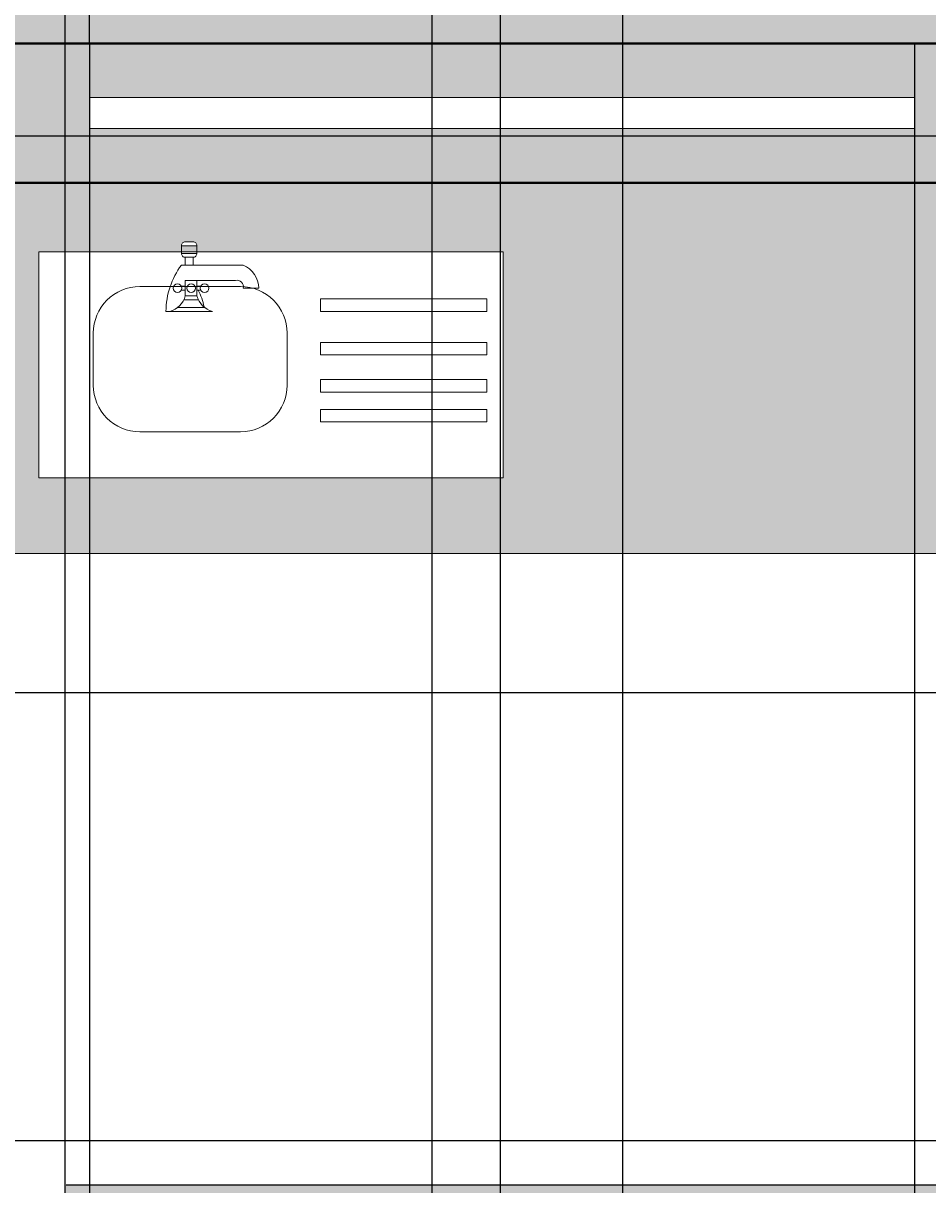
# Model space of a CAD drawing. Units: inches. Extents: x 818 to 1898, y 976 to 2364.
# Tile 85 of 96: x 1481 to 1539, y 1979 to 2054. Entities that reach past the tile are written whole.
import ezdxf

# ---------------------------------------------------------------- set-up
doc = ezdxf.new("R2010")
doc.units = ezdxf.units.IN
doc.header["$LTSCALE"] = 5
doc.header["$MEASUREMENT"] = 0
for name, color, linetype, lineweight in [('A-ANNO-DIMS', 2, 'Continuous', 18), ('A-FLOR-CASE', 8, 'Continuous', 18), ('A-FLOR-FIXT', 9, 'Continuous', 18), ('A-FURN-PATT', 8, 'Continuous', 9), ('A-GLAZ', 4, 'Continuous', 18), ('A-WALL', 7, 'Continuous', 40)]:
    doc.layers.add(name, color=color, linetype=linetype, lineweight=lineweight)
for name, color, linetype, lineweight, true_color in [('A-GLAZ-PATT', 141, 'Continuous', 9, 0xadddf7), ('A-WALL-PATT', 251, 'Continuous', 13, 0x636466), ('L-PLNT-PATT', 114, 'Continuous', 9, 0x139b48)]:
    doc.layers.add(name, color=color, linetype=linetype, lineweight=lineweight, true_color=true_color)
doc.styles.get("Standard").update_dxf_attribs({"font": 'arial.ttf'})
doc.dimstyles.get("Standard").update_dxf_attribs({"dimtxt": 0.18, "dimasz": 0.18, "dimexe": 0.18, "dimexo": 0.0625, "dimgap": 0.09, "dimtad": 0, "dimtih": 1, "dimtoh": 1, "dimdec": 4, "dimzin": 0, "dimdsep": 46, "dimtxsty": 'Standard', "dimcen": 0.09, "dimadec": 0, "dimazin": 0, "dimtfac": 1, "dimtdec": 4, "dimtofl": 0, "dimtmove": 0, "dimatfit": 3, "dimfxl": 1, "dimtolj": 1, "dimtzin": 0, "dimarcsym": 0})

# ---------------------------------------------------------------- blocks, each defined once
blk = doc.blocks.new('Faucet - Bathroom side')
for p, q in [((-0.625, 4.25), (0.375, 4.25)), ((0.375, 3.75), (-0.625, 3.75)), ((-0.375, 3), (-0.375, 3.5)), ((0.125, 3.5), (0.125, 3)), ((-0.625, 3), (3.375, 3)), ((-0.375, 1.625), (-0.625, 1.625)), ((2.875, 2), (0.375, 2)), ((0.375, 1.625), (0.625, 1.625)), ((-0.375, 1.375), (-0.625, 1.375)), ((0.375, 1.375), (0.625, 1.375)), ((4.375, 1.5), (3.375, 1.5)), ((-1.625, 0), (-1.375, 0)), ((-1.375, 0), (1.375, 0)), ((-0.88366, 0.25), (0.88424, 0.25)), ((0.48078, 0.75), (-0.47286, 0.75))]:
    blk.add_line(p, q)
for points in [[(-0.625, 3.75), (-0.625, 4.25)], [(-0.375, 4.5), (0.125, 4.5)], [(0.375, 4.25), (0.375, 3.75)], [(0.125, 3.5), (-0.375, 3.5)]]:
    blk.add_lwpolyline(points)
blk.add_lwpolyline([(-0.375, 1), (-0.375, 2), (0.375, 2), (0.375, 1)], close=True)
for centre in [(-0.875, 1.5), (0, 1.5), (0.875, 1.5)]:
    blk.add_circle(centre, 0.27951)
for centre, radius, start, end in [((-0.38253, 4.2575), 0.24259, 88.22243, 181.7776), ((0.13252, 4.2575), 0.24259, 358.2224, 91.77757), ((-0.38253, 3.7424), 0.24259, 178.2224, 271.7776), ((0.13252, 3.7424), 0.24259, 268.2224, 1.777565), ((3.45929, -0.0281), 5.08436, 143.4467, 179.6834), ((2.70708, 1.4714), 1.66816, 0.9827695, 66.39737), ((2.96867, 1.5936), 0.41699, 347.0192, 102.9808), ((-1.75, 1.375), 1.42522, 285.2551, 344.7449), ((1.75, 1.375), 1.42522, 195.2551, 254.7449), ((-2.49562, -0.286), 3.38273, 9.709485, 29.48735)]:
    blk.add_arc(centre, radius, start, end)
blk = doc.blocks.new('*D73')
at = {"layer": 'A-ANNO-DIMS', "color": 0, "lineweight": -2, "ltscale": 5, "transparency": 16777216}
for p, q in [((1590.663, 2011.078), (818.026, 2011.078)), ((818.206, 2010.898), (818.206, 1996.76)), ((818.206, 1982.258), (818.206, 1996.396)), ((1590.663, 1982.078), (818.026, 1982.078))]:
    blk.add_line(p, q, dxfattribs=at)
at = {"layer": 'A-ANNO-DIMS', "color": 0, "ltscale": 5, "transparency": 16777216}
for points in [[(818.176, 2010.898), (818.236, 2010.898), (818.206, 2011.078)], [(818.176, 1982.258), (818.236, 1982.258), (818.206, 1982.078)]]:
    blk.add_solid(points, dxfattribs=at)
at = {"layer": 'Defpoints', "color": 0, "ltscale": 5, "transparency": 16777216}
for p in [(818.206, 2011.078), (1590.725, 2011.078), (1590.725, 1982.078)]:
    blk.add_point(p, dxfattribs=at)
at = {"layer": 'A-ANNO-DIMS', "color": 0, "ltscale": 5, "transparency": 16777216, "insert": (818.206, 1996.578), "char_height": 0.18, "attachment_point": 5}
blk.add_mtext('\\A1;29', dxfattribs=at)
blk = doc.blocks.new('*D85')
at = {"layer": 'A-ANNO-DIMS', "color": 0, "lineweight": -2, "ltscale": 5, "transparency": 16777216}
for p, q in [((1258.788, 2053.078), (1897.916, 2053.078)), ((1897.736, 2052.898), (1897.736, 1876.76)), ((1897.736, 1700.258), (1897.736, 1876.396)), ((1258.788, 1700.078), (1897.916, 1700.078))]:
    blk.add_line(p, q, dxfattribs=at)
at = {"layer": 'A-ANNO-DIMS', "color": 0, "ltscale": 5, "transparency": 16777216}
for points in [[(1897.706, 2052.898), (1897.766, 2052.898), (1897.736, 2053.078)], [(1897.706, 1700.258), (1897.766, 1700.258), (1897.736, 1700.078)]]:
    blk.add_solid(points, dxfattribs=at)
at = {"layer": 'Defpoints', "color": 0, "ltscale": 5, "transparency": 16777216}
for p in [(1258.725, 2053.078), (1897.736, 2053.078), (1258.725, 1700.078)]:
    blk.add_point(p, dxfattribs=at)
at = {"layer": 'A-ANNO-DIMS', "color": 0, "ltscale": 5, "transparency": 16777216, "insert": (1897.736, 1876.578), "char_height": 0.18, "attachment_point": 5}
blk.add_mtext('\\A1;353', dxfattribs=at)
blk = doc.blocks.new('*D86')
at = {"layer": 'A-ANNO-DIMS', "color": 0, "lineweight": -2, "ltscale": 5, "transparency": 16777216}
for p, q in [((1258.725, 2053.141), (1258.725, 2363.873)), ((1258.905, 2363.693), (1486.433, 2363.693)), ((1714.545, 2363.693), (1487.018, 2363.693)), ((1714.725, 2053.141), (1714.725, 2363.873))]:
    blk.add_line(p, q, dxfattribs=at)
at = {"layer": 'A-ANNO-DIMS', "color": 0, "ltscale": 5, "transparency": 16777216}
for points in [[(1258.905, 2363.723), (1258.905, 2363.663), (1258.725, 2363.693)], [(1714.545, 2363.723), (1714.545, 2363.663), (1714.725, 2363.693)]]:
    blk.add_solid(points, dxfattribs=at)
at = {"layer": 'Defpoints', "color": 0, "ltscale": 5, "transparency": 16777216}
for p in [(1714.725, 2363.693), (1258.725, 2053.078), (1714.725, 2053.078)]:
    blk.add_point(p, dxfattribs=at)
at = {"layer": 'A-ANNO-DIMS', "color": 0, "ltscale": 5, "transparency": 16777216, "insert": (1486.725, 2363.693), "char_height": 0.18, "attachment_point": 5}
blk.add_mtext('\\A1;456', dxfattribs=at)
blk = doc.blocks.new('*D100')
at = {"layer": 'A-ANNO-DIMS', "color": 0, "lineweight": -2, "ltscale": 5, "transparency": 16777216}
for p, q in [((1449.82, 1071.118), (1449.82, 2363.873)), ((1450, 2363.693), (1478.165, 2363.693)), ((1507.118, 2363.693), (1478.953, 2363.693)), ((1507.298, 1071.118), (1507.298, 2363.873))]:
    blk.add_line(p, q, dxfattribs=at)
at = {"layer": 'A-ANNO-DIMS', "color": 0, "ltscale": 5, "transparency": 16777216}
for points in [[(1450, 2363.723), (1450, 2363.663), (1449.82, 2363.693)], [(1507.118, 2363.723), (1507.118, 2363.663), (1507.298, 2363.693)]]:
    blk.add_solid(points, dxfattribs=at)
at = {"layer": 'Defpoints', "color": 0, "ltscale": 5, "transparency": 16777216}
for p in [(1507.298, 2363.693), (1449.82, 1071.055), (1507.298, 1071.055)]:
    blk.add_point(p, dxfattribs=at)
at = {"layer": 'A-ANNO-DIMS', "color": 0, "ltscale": 5, "transparency": 16777216, "insert": (1478.559, 2363.693), "char_height": 0.18, "attachment_point": 5}
blk.add_mtext('\\A1;57.48', dxfattribs=at)
blk = doc.blocks.new('*D101')
at = {"layer": 'A-ANNO-DIMS', "color": 0, "lineweight": -2, "ltscale": 5, "transparency": 16777216}
for p, q in [((1507.298, 1071.118), (1507.298, 2363.873)), ((1507.478, 2363.693), (1535.997, 2363.693)), ((1565.303, 2363.693), (1536.785, 2363.693)), ((1565.483, 1071.118), (1565.483, 2363.873))]:
    blk.add_line(p, q, dxfattribs=at)
at = {"layer": 'A-ANNO-DIMS', "color": 0, "ltscale": 5, "transparency": 16777216}
for points in [[(1507.478, 2363.723), (1507.478, 2363.663), (1507.298, 2363.693)], [(1565.303, 2363.723), (1565.303, 2363.663), (1565.483, 2363.693)]]:
    blk.add_solid(points, dxfattribs=at)
at = {"layer": 'Defpoints', "color": 0, "ltscale": 5, "transparency": 16777216}
for p in [(1565.483, 2363.693), (1507.298, 1071.055), (1565.483, 1071.055)]:
    blk.add_point(p, dxfattribs=at)
at = {"layer": 'A-ANNO-DIMS', "color": 0, "ltscale": 5, "transparency": 16777216, "insert": (1536.391, 2363.693), "char_height": 0.18, "attachment_point": 5}
blk.add_mtext('\\A1;58.19', dxfattribs=at)
blk = doc.blocks.new('*D161')
at = {"layer": 'A-ANNO-DIMS', "color": 0, "lineweight": -2, "ltscale": 5, "transparency": 16777216}
for p, q in [((1429.225, 1876.141), (1429.225, 2363.873)), ((1429.405, 2363.693), (1509.589, 2363.693)), ((1590.545, 2363.693), (1510.361, 2363.693)), ((1590.725, 1876.141), (1590.725, 2363.873))]:
    blk.add_line(p, q, dxfattribs=at)
at = {"layer": 'A-ANNO-DIMS', "color": 0, "ltscale": 5, "transparency": 16777216}
for points in [[(1429.405, 2363.723), (1429.405, 2363.663), (1429.225, 2363.693)], [(1590.545, 2363.723), (1590.545, 2363.663), (1590.725, 2363.693)]]:
    blk.add_solid(points, dxfattribs=at)
at = {"layer": 'Defpoints', "color": 0, "ltscale": 5, "transparency": 16777216}
for p in [(1590.725, 2363.693), (1429.225, 1876.078), (1590.725, 1876.078)]:
    blk.add_point(p, dxfattribs=at)
at = {"layer": 'A-ANNO-DIMS', "color": 0, "ltscale": 5, "transparency": 16777216, "insert": (1509.975, 2363.693), "char_height": 0.18, "attachment_point": 5}
blk.add_mtext('\\A1;161.5', dxfattribs=at)
blk = doc.blocks.new('*D207')
at = {"layer": 'A-ANNO-DIMS', "color": 0, "lineweight": -2, "ltscale": 5, "transparency": 16777216}
for p, q in [((1590.663, 2044.078), (818.026, 2044.078)), ((818.206, 2043.898), (818.206, 2027.76)), ((818.206, 2011.258), (818.206, 2027.396)), ((1590.663, 2011.078), (818.026, 2011.078))]:
    blk.add_line(p, q, dxfattribs=at)
at = {"layer": 'A-ANNO-DIMS', "color": 0, "ltscale": 5, "transparency": 16777216}
for points in [[(818.176, 2043.898), (818.236, 2043.898), (818.206, 2044.078)], [(818.176, 2011.258), (818.236, 2011.258), (818.206, 2011.078)]]:
    blk.add_solid(points, dxfattribs=at)
at = {"layer": 'Defpoints', "color": 0, "ltscale": 5, "transparency": 16777216}
for p in [(818.206, 2044.078), (1590.725, 2044.078), (1590.725, 2011.078)]:
    blk.add_point(p, dxfattribs=at)
at = {"layer": 'A-ANNO-DIMS', "color": 0, "ltscale": 5, "transparency": 16777216, "insert": (818.206, 2027.578), "char_height": 0.18, "attachment_point": 5}
blk.add_mtext('\\A1;33', dxfattribs=at)
blk = doc.blocks.new('*D238')
at = {"layer": 'A-ANNO-DIMS', "color": 0, "lineweight": -2, "ltscale": 5, "transparency": 16777216}
for p, q in [((1483.545, 1948.723), (1483.545, 2363.873)), ((1483.725, 2363.693), (1516.384, 2363.693)), ((1549.831, 2363.693), (1517.172, 2363.693)), ((1550.011, 1948.723), (1550.011, 2363.873))]:
    blk.add_line(p, q, dxfattribs=at)
at = {"layer": 'A-ANNO-DIMS', "color": 0, "ltscale": 5, "transparency": 16777216}
for points in [[(1483.725, 2363.723), (1483.725, 2363.663), (1483.545, 2363.693)], [(1549.831, 2363.723), (1549.831, 2363.663), (1550.011, 2363.693)]]:
    blk.add_solid(points, dxfattribs=at)
at = {"layer": 'Defpoints', "color": 0, "ltscale": 5, "transparency": 16777216}
for p in [(1550.011, 2363.693), (1483.545, 1948.66), (1550.011, 1948.66)]:
    blk.add_point(p, dxfattribs=at)
at = {"layer": 'A-ANNO-DIMS', "color": 0, "ltscale": 5, "transparency": 16777216, "insert": (1516.778, 2363.693), "char_height": 0.18, "attachment_point": 5}
blk.add_mtext('\\A1;66.47', dxfattribs=at)
blk = doc.blocks.new('*D239')
at = {"layer": 'A-ANNO-DIMS', "color": 0, "lineweight": -2, "ltscale": 5, "transparency": 16777216}
for p, q in [((1483.608, 1979.244), (1897.916, 1979.244)), ((1897.736, 1979.064), (1897.736, 1964.134)), ((1897.736, 1948.84), (1897.736, 1963.77)), ((1483.608, 1948.66), (1897.916, 1948.66))]:
    blk.add_line(p, q, dxfattribs=at)
at = {"layer": 'A-ANNO-DIMS', "color": 0, "ltscale": 5, "transparency": 16777216}
for points in [[(1897.706, 1979.064), (1897.766, 1979.064), (1897.736, 1979.244)], [(1897.706, 1948.84), (1897.766, 1948.84), (1897.736, 1948.66)]]:
    blk.add_solid(points, dxfattribs=at)
at = {"layer": 'Defpoints', "color": 0, "ltscale": 5, "transparency": 16777216}
for p in [(1483.545, 1979.244), (1897.736, 1979.244), (1483.545, 1948.66)]:
    blk.add_point(p, dxfattribs=at)
at = {"layer": 'A-ANNO-DIMS', "color": 0, "ltscale": 5, "transparency": 16777216, "insert": (1897.736, 1963.952), "char_height": 0.18, "attachment_point": 5}
blk.add_mtext('\\A1;30.584', dxfattribs=at)
blk = doc.blocks.new('*D243')
at = {"layer": 'A-ANNO-DIMS', "color": 0, "lineweight": -2, "ltscale": 5, "transparency": 16777216}
for p, q in [((1451.77, 2020.016), (1451.77, 975.663)), ((1590.725, 2020.016), (1590.725, 975.663)), ((1451.95, 975.843), (1520.792, 975.843)), ((1590.545, 975.843), (1521.703, 975.843))]:
    blk.add_line(p, q, dxfattribs=at)
at = {"layer": 'A-ANNO-DIMS', "color": 0, "ltscale": 5, "transparency": 16777216}
for points in [[(1451.95, 975.873), (1451.95, 975.813), (1451.77, 975.843)], [(1590.545, 975.873), (1590.545, 975.813), (1590.725, 975.843)]]:
    blk.add_solid(points, dxfattribs=at)
at = {"layer": 'Defpoints', "color": 0, "ltscale": 5, "transparency": 16777216}
for p in [(1451.77, 2020.078), (1590.725, 2020.078), (1590.725, 975.843)]:
    blk.add_point(p, dxfattribs=at)
at = {"layer": 'A-ANNO-DIMS', "color": 0, "ltscale": 5, "transparency": 16777216, "insert": (1521.247, 975.843), "char_height": 0.18, "attachment_point": 5}
blk.add_mtext('\\A1;138.96', dxfattribs=at)
blk = doc.blocks.new('*D244')
at = {"layer": 'A-ANNO-DIMS', "color": 0, "lineweight": -2, "ltscale": 5, "transparency": 16777216}
for p, q in [((1519.641, 1900.141), (1519.641, 2363.873)), ((1519.821, 2363.693), (1554.79, 2363.693)), ((1590.545, 2363.693), (1555.576, 2363.693)), ((1590.725, 1900.141), (1590.725, 2363.873))]:
    blk.add_line(p, q, dxfattribs=at)
at = {"layer": 'A-ANNO-DIMS', "color": 0, "ltscale": 5, "transparency": 16777216}
for points in [[(1519.821, 2363.723), (1519.821, 2363.663), (1519.641, 2363.693)], [(1590.545, 2363.723), (1590.545, 2363.663), (1590.725, 2363.693)]]:
    blk.add_solid(points, dxfattribs=at)
at = {"layer": 'Defpoints', "color": 0, "ltscale": 5, "transparency": 16777216}
for p in [(1590.725, 2363.693), (1519.641, 1900.078), (1590.725, 1900.078)]:
    blk.add_point(p, dxfattribs=at)
at = {"layer": 'A-ANNO-DIMS', "color": 0, "ltscale": 5, "transparency": 16777216, "insert": (1555.183, 2363.693), "char_height": 0.18, "attachment_point": 5}
blk.add_mtext('\\A1;71.08', dxfattribs=at)
blk = doc.blocks.new('*D253')
at = {"layer": 'A-ANNO-DIMS', "color": 0, "lineweight": -2, "ltscale": 5, "transparency": 16777216}
for p, q in [((1485.122, 2053.016), (1485.122, 975.663)), ((1538.516, 2053.016), (1538.516, 975.663)), ((1485.302, 975.843), (1511.425, 975.843)), ((1538.336, 975.843), (1512.212, 975.843))]:
    blk.add_line(p, q, dxfattribs=at)
at = {"layer": 'A-ANNO-DIMS', "color": 0, "ltscale": 5, "transparency": 16777216}
for points in [[(1485.302, 975.873), (1485.302, 975.813), (1485.122, 975.843)], [(1538.336, 975.873), (1538.336, 975.813), (1538.516, 975.843)]]:
    blk.add_solid(points, dxfattribs=at)
at = {"layer": 'Defpoints', "color": 0, "ltscale": 5, "transparency": 16777216}
for p in [(1485.122, 2053.078), (1538.516, 2053.078), (1538.516, 975.843)]:
    blk.add_point(p, dxfattribs=at)
at = {"layer": 'A-ANNO-DIMS', "color": 0, "ltscale": 5, "transparency": 16777216, "insert": (1511.819, 975.843), "char_height": 0.18, "attachment_point": 5}
blk.add_mtext('\\A1;53.39', dxfattribs=at)
blk = doc.blocks.new('*D258')
at = {"layer": 'A-ANNO-DIMS', "color": 0, "lineweight": -2, "ltscale": 5, "transparency": 16777216}
for p, q in [((1422.02, 2053.141), (1422.02, 2363.873)), ((1422.2, 2363.693), (1453.264, 2363.693)), ((1484.942, 2363.693), (1453.878, 2363.693)), ((1485.122, 2053.141), (1485.122, 2363.873))]:
    blk.add_line(p, q, dxfattribs=at)
at = {"layer": 'A-ANNO-DIMS', "color": 0, "ltscale": 5, "transparency": 16777216}
for points in [[(1422.2, 2363.723), (1422.2, 2363.663), (1422.02, 2363.693)], [(1484.942, 2363.723), (1484.942, 2363.663), (1485.122, 2363.693)]]:
    blk.add_solid(points, dxfattribs=at)
at = {"layer": 'Defpoints', "color": 0, "ltscale": 5, "transparency": 16777216}
for p in [(1485.122, 2363.693), (1422.02, 2053.078), (1485.122, 2053.078)]:
    blk.add_point(p, dxfattribs=at)
at = {"layer": 'A-ANNO-DIMS', "color": 0, "ltscale": 5, "transparency": 16777216, "insert": (1453.571, 2363.693), "char_height": 0.18, "attachment_point": 5}
blk.add_mtext('\\A1;63.1', dxfattribs=at)
blk = doc.blocks.new('*D266')
at = {"layer": 'A-ANNO-DIMS', "color": 0, "lineweight": -2, "ltscale": 5, "transparency": 16777216}
for p, q in [((1780.439, 2053.078), (818.026, 2053.078)), ((818.206, 2052.898), (818.206, 2050.26)), ((818.206, 2047.258), (818.206, 2049.896)), ((1780.439, 2047.078), (818.026, 2047.078))]:
    blk.add_line(p, q, dxfattribs=at)
at = {"layer": 'A-ANNO-DIMS', "color": 0, "ltscale": 5, "transparency": 16777216}
for points in [[(818.176, 2052.898), (818.236, 2052.898), (818.206, 2053.078)], [(818.176, 2047.258), (818.236, 2047.258), (818.206, 2047.078)]]:
    blk.add_solid(points, dxfattribs=at)
at = {"layer": 'Defpoints', "color": 0, "ltscale": 5, "transparency": 16777216}
for p in [(1780.502, 2053.078), (818.206, 2047.078), (1780.502, 2047.078)]:
    blk.add_point(p, dxfattribs=at)
at = {"layer": 'A-ANNO-DIMS', "color": 0, "ltscale": 5, "transparency": 16777216, "insert": (818.206, 2050.078), "char_height": 0.18, "attachment_point": 5}
blk.add_mtext('\\A1;6', dxfattribs=at)
blk = doc.blocks.new('*D281')
at = {"layer": 'A-ANNO-DIMS', "color": 0, "lineweight": -2, "ltscale": 5, "transparency": 16777216}
for p, q in [((1250.303, 1913.703), (1250.303, 2363.873)), ((1250.483, 2363.693), (1420.121, 2363.693)), ((1590.545, 2363.693), (1420.907, 2363.693)), ((1590.725, 2011.141), (1590.725, 2363.873))]:
    blk.add_line(p, q, dxfattribs=at)
at = {"layer": 'A-ANNO-DIMS', "color": 0, "ltscale": 5, "transparency": 16777216}
for points in [[(1250.483, 2363.723), (1250.483, 2363.663), (1250.303, 2363.693)], [(1590.545, 2363.723), (1590.545, 2363.663), (1590.725, 2363.693)]]:
    blk.add_solid(points, dxfattribs=at)
at = {"layer": 'Defpoints', "color": 0, "ltscale": 5, "transparency": 16777216}
for p in [(1590.725, 2363.693), (1590.725, 2011.078), (1250.303, 1913.64)]:
    blk.add_point(p, dxfattribs=at)
at = {"layer": 'A-ANNO-DIMS', "color": 0, "ltscale": 5, "transparency": 16777216, "insert": (1420.514, 2363.693), "char_height": 0.18, "attachment_point": 5}
blk.add_mtext('\\A1;340.4', dxfattribs=at)
blk = doc.blocks.new('*D282')
at = {"layer": 'A-ANNO-DIMS', "color": 0, "lineweight": -2, "ltscale": 5, "transparency": 16777216}
for p, q in [((1422.083, 2081.188), (1897.916, 2081.188)), ((1897.736, 2081.008), (1897.736, 1884.315)), ((1897.736, 1687.258), (1897.736, 1883.951)), ((1463.788, 1687.078), (1897.916, 1687.078))]:
    blk.add_line(p, q, dxfattribs=at)
at = {"layer": 'A-ANNO-DIMS', "color": 0, "ltscale": 5, "transparency": 16777216}
for points in [[(1897.706, 2081.008), (1897.766, 2081.008), (1897.736, 2081.188)], [(1897.706, 1687.258), (1897.766, 1687.258), (1897.736, 1687.078)]]:
    blk.add_solid(points, dxfattribs=at)
at = {"layer": 'Defpoints', "color": 0, "ltscale": 5, "transparency": 16777216}
for p in [(1422.02, 2081.188), (1897.736, 2081.188), (1463.725, 1687.078)]:
    blk.add_point(p, dxfattribs=at)
at = {"layer": 'A-ANNO-DIMS', "color": 0, "ltscale": 5, "transparency": 16777216, "insert": (1897.736, 1884.133), "char_height": 0.18, "attachment_point": 5}
blk.add_mtext('\\A1;394.1', dxfattribs=at)
blk = doc.blocks.new('*D288')
at = {"layer": 'A-ANNO-DIMS', "color": 0, "lineweight": -2, "ltscale": 5, "transparency": 16777216}
for p, q in [((1422.876, 1742.674), (1422.876, 2363.873)), ((1423.056, 2363.693), (1466.906, 2363.693)), ((1511.545, 2363.693), (1467.695, 2363.693)), ((1511.725, 1716.108), (1511.725, 2363.873))]:
    blk.add_line(p, q, dxfattribs=at)
at = {"layer": 'A-ANNO-DIMS', "color": 0, "ltscale": 5, "transparency": 16777216}
for points in [[(1423.056, 2363.723), (1423.056, 2363.663), (1422.876, 2363.693)], [(1511.545, 2363.723), (1511.545, 2363.663), (1511.725, 2363.693)]]:
    blk.add_solid(points, dxfattribs=at)
at = {"layer": 'Defpoints', "color": 0, "ltscale": 5, "transparency": 16777216}
for p in [(1511.725, 2363.693), (1422.876, 1742.611), (1511.725, 1716.045)]:
    blk.add_point(p, dxfattribs=at)
at = {"layer": 'A-ANNO-DIMS', "color": 0, "ltscale": 5, "transparency": 16777216, "insert": (1467.3, 2363.693), "char_height": 0.18, "attachment_point": 5}
blk.add_mtext('\\A1;88.85', dxfattribs=at)

msp = doc.modelspace()

# ---------------------------------------------------------------- hatches: boundary and pattern name
at = {"layer": 'A-FURN-PATT', "ltscale": 5}
h = msp.add_hatch(color=256, dxfattribs=at)
h.dxf.hatch_style = 1
h.paths.add_polyline_path([(1341.9997, 1981.5338), (1317.9034, 2001.8247), (1314.2595, 2001.8247), (1314.2595, 2004.893), (1310.1046, 2008.3917), (1303.9314, 2008.3917), (1303.9314, 1953.0408), (1308.1629, 1953.0408), (1314.2595, 1958.1746), (1314.2595, 1959.6079), (1315.9616, 1959.6079)])
h.paths.add_polyline_path([(1341.9997, 1981.5338), (1315.9616, 1959.6079), (1336.7936, 1959.6079), (1336.7936, 1953.0408), (1345.3966, 1953.0408), (1345.3966, 1959.6079), (1368.0379, 1959.6079)])
h.paths.add_polyline_path([(1402.518, 2008.3917), (1398.8475, 2008.3917), (1398.8475, 2001.8247), (1376.3134, 2001.8247), (1376.3134, 2008.3917), (1373.8948, 2008.3917), (1367.9307, 2003.3695), (1367.9307, 2001.8247), (1366.0961, 2001.8247), (1341.9997, 1981.5338), (1368.0379, 1959.6079), (1375.8366, 1953.0408), (1376.3134, 1953.0408), (1376.3134, 1959.6079), (1398.8475, 1959.6079), (1398.8475, 1953.0408), (1402.518, 1953.0408)])
h.paths.add_polyline_path([(1366.0961, 2001.8247), (1345.3966, 2001.8247), (1345.3966, 2008.3917), (1336.7936, 2008.3917), (1336.7936, 2001.8247), (1317.9034, 2001.8247), (1341.9997, 1981.5338)])
h.paths.add_polyline_path([(1336.7936, 1959.6079), (1315.9616, 1959.6079), (1314.2595, 1958.1746), (1314.2595, 1953.0408), (1336.7936, 1953.0408)], flags=17)
h.paths.add_polyline_path([(1367.9307, 1959.6079), (1345.3966, 1959.6079), (1345.3966, 1953.0408), (1367.9307, 1953.0408)], flags=17)
h.paths.add_polyline_path([(1398.8475, 1959.6079), (1376.3134, 1959.6079), (1376.3134, 1953.0408), (1398.8475, 1953.0408)], flags=17)
h.paths.add_polyline_path([(1368.0379, 1959.6079), (1367.9307, 1959.6079), (1367.9307, 1953.0408), (1375.8366, 1953.0408)], flags=17)
h.paths.add_polyline_path([(1314.2595, 1958.1746), (1308.1629, 1953.0408), (1314.2595, 1953.0408)], flags=17)
h.paths.add_polyline_path([(1315.9616, 1959.6079), (1314.2595, 1959.6079), (1314.2595, 1958.1746)], flags=16)
h.paths.add_polyline_path([(1314.2595, 2008.3917), (1310.1046, 2008.3917), (1314.2595, 2004.893)], flags=17)
h.paths.add_polyline_path([(1336.7936, 2008.3917), (1314.2595, 2008.3917), (1314.2595, 2004.893), (1317.9034, 2001.8247), (1336.7936, 2001.8247)], flags=17)
h.paths.add_polyline_path([(1314.2595, 2004.893), (1314.2595, 2001.8247), (1317.9034, 2001.8247)], flags=16)
h.paths.add_polyline_path([(1367.9307, 2008.3917), (1345.3966, 2008.3917), (1345.3966, 2001.8247), (1366.0961, 2001.8247), (1367.9307, 2003.3695)], flags=17)
h.paths.add_polyline_path([(1398.8475, 2008.3917), (1376.3134, 2008.3917), (1376.3134, 2001.8247), (1398.8475, 2001.8247)], flags=17)
h.paths.add_polyline_path([(1373.8948, 2008.3917), (1367.9307, 2008.3917), (1367.9307, 2003.3695)], flags=17)
h.paths.add_polyline_path([(1367.9307, 2003.3695), (1366.0961, 2001.8247), (1367.9307, 2001.8247)], flags=16)
h.paths.add_polyline_path([(1546.1595, 2044.0782), (1451.7698, 2044.0782), (1451.7698, 2020.0782), (1546.1595, 2020.0782)])
h.paths.add_polyline_path([(1492.0729, 2040.001, 0.431429), (1491.8238, 2040.251), (1491.3087, 2040.251, 0.415217), (1491.0729, 2040.001)], flags=16)
h.paths.add_polyline_path([(1481.8346, 2039.6036), (1511.886, 2039.6036), (1511.886, 2024.9917), (1481.8346, 2024.9917)], flags=16)
h.paths.add_polyline_path([(1491.0729, 2039.4857), (1491.0729, 2039.501), (1492.0729, 2039.501, -0.4117484), (1491.8401, 2039.251), (1491.8229, 2039.251), (1491.8229, 2039.2509, 0.4325918), (1492.0729, 2039.501), (1491.0729, 2039.501, 0.432604), (1491.3229, 2039.2509), (1491.3229, 2039.251), (1491.325, 2039.251, -0.4165823)], flags=0)
h.paths.add_polyline_path([(1485.3701, 2030.9622), (1485.3701, 2034.3556, -0.4142136), (1488.3701, 2037.3556), (1490.3421, 2037.3556, -0.0779193), (1491.0729, 2038.751), (1495.0729, 2038.751, -0.3148679), (1496.07, 2037.1201, -0.3016609), (1497.9049, 2034.3556), (1497.9049, 2030.9622, -0.4142136), (1494.9049, 2027.9622), (1488.3701, 2027.9622, -0.4142136)], flags=0)
h.paths.add_polyline_path([(1490.3229, 2035.751, 0.2655648), (1491.3229, 2036.751), (1491.3229, 2037.126), (1491.0729, 2037.126, -0.7914183), (1490.5434, 2037.251, -0.7914183), (1491.0729, 2037.376), (1491.3229, 2037.376), (1491.3229, 2037.751), (1492.0729, 2037.751), (1492.0729, 2037.376), (1492.3229, 2037.376, -0.7914183), (1492.8524, 2037.251, -0.7914183), (1492.3229, 2037.126), (1492.1491, 2037.126, -0.0866263), (1492.5376, 2036.0294, 0.1070481), (1493.0729, 2035.751), (1490.3229, 2035.751)], flags=0)
h.paths.add_polyline_path([(1491.9774, 2037.251, -1), (1491.4184, 2037.251, -1)], flags=0)
h.paths.add_polyline_path([(1500.0743, 2028.6045), (1500.0743, 2029.4074), (1510.8414, 2029.4074), (1510.8414, 2028.6045)], flags=0)
h.paths.add_polyline_path([(1500.0743, 2030.5314), (1500.0743, 2031.3342), (1510.8414, 2031.3342), (1510.8414, 2030.5314)], flags=0)
h.paths.add_polyline_path([(1500.0743, 2032.94), (1500.0743, 2033.7428), (1510.8414, 2033.7428), (1510.8414, 2032.94)], flags=0)
h.paths.add_polyline_path([(1500.0743, 2035.7499), (1500.0743, 2036.5528), (1510.8414, 2036.5528), (1510.8414, 2035.7499)], flags=0)
h.paths.add_polyline_path([(1590.7251, 2044.0782), (1576.1595, 2044.0782), (1576.1595, 2020.0782), (1590.7251, 2020.0782)])
h.paths.add_polyline_path([(1668.4429, 2044.0782), (1599.7252, 2044.0782), (1599.7252, 2020.0782), (1668.4429, 2020.0782)])
h.paths.add_polyline_path([(1621.2588, 2040.001, 0.431429), (1621.0097, 2040.251), (1620.4946, 2040.251, 0.415217), (1620.2588, 2040.001)], flags=16)
h.paths.add_polyline_path([(1611.0205, 2024.9917), (1611.0205, 2039.6036), (1641.0719, 2039.6036), (1641.0719, 2024.9917)], flags=16)
h.paths.add_polyline_path([(1620.2588, 2039.4857), (1620.2588, 2039.501), (1621.2588, 2039.501, -0.4117484), (1621.026, 2039.251), (1621.0088, 2039.251), (1621.0088, 2039.2509, 0.4325918), (1621.2588, 2039.501), (1620.2588, 2039.501, 0.432604), (1620.5088, 2039.2509), (1620.5088, 2039.251), (1620.5109, 2039.251, -0.4165823)], flags=0)
h.paths.add_polyline_path([(1614.556, 2030.9622), (1614.556, 2034.3556, -0.4142136), (1617.556, 2037.3556), (1619.528, 2037.3556, -0.0779193), (1620.2588, 2038.751), (1624.2588, 2038.751, -0.3148679), (1625.2559, 2037.1201, -0.3016609), (1627.0908, 2034.3556), (1627.0908, 2030.9622, -0.4142136), (1624.0908, 2027.9622), (1617.556, 2027.9622, -0.4142136)], flags=0)
h.paths.add_polyline_path([(1619.5088, 2035.751, 0.2655648), (1620.5088, 2036.751), (1620.5088, 2037.126), (1620.2588, 2037.126, -0.7914183), (1619.7293, 2037.251, -0.7914183), (1620.2588, 2037.376), (1620.5088, 2037.376), (1620.5088, 2037.751), (1621.2588, 2037.751), (1621.2588, 2037.376), (1621.5088, 2037.376, -0.7914183), (1622.0383, 2037.251, -0.7914183), (1621.5088, 2037.126), (1621.335, 2037.126, -0.0866263), (1621.7235, 2036.0294, 0.1070481), (1622.2588, 2035.751), (1619.5088, 2035.751)], flags=0)
h.paths.add_polyline_path([(1620.6043, 2037.251, -1), (1621.1633, 2037.251, -1)], flags=0)
h.paths.add_polyline_path([(1629.2602, 2028.6045), (1629.2602, 2029.4074), (1640.0273, 2029.4074), (1640.0273, 2028.6045)], flags=0)
h.paths.add_polyline_path([(1629.2602, 2030.5314), (1629.2602, 2031.3342), (1640.0273, 2031.3342), (1640.0273, 2030.5314)], flags=0)
h.paths.add_polyline_path([(1629.2602, 2032.94), (1629.2602, 2033.7428), (1640.0273, 2033.7428), (1640.0273, 2032.94)], flags=0)
h.paths.add_polyline_path([(1629.2602, 2035.7499), (1629.2602, 2036.5528), (1640.0273, 2036.5528), (1640.0273, 2035.7499)], flags=0)
h.paths.add_polyline_path([(1705.7252, 2044.0782), (1698.4429, 2044.0782), (1698.4429, 2020.0782), (1705.7252, 2020.0782)])
h.paths.add_polyline_path([(1705.7252, 1972.0782), (1599.7252, 1972.0782), (1599.7252, 1948.0782), (1705.7252, 1948.0782)])
h.paths.add_polyline_path([(1550.0109, 1979.2444), (1483.5451, 1979.2444), (1483.5451, 1948.6602), (1550.0109, 1948.6602)])
h.paths.add_polyline_path([(1490.2586, 1948.6602), (1488.2586, 1948.6602), (1488.2586, 1941.1742, 0.4142136), (1491.2586, 1938.1742), (1500.7446, 1938.1742, -0.4142136)])
h.paths.add_polyline_path([(1513.2306, 1941.1742), (1513.2306, 1948.6602), (1511.2306, 1948.6602, -0.4142136), (1500.7446, 1938.1742), (1510.2306, 1938.1742, 0.4142136)])
h.paths.add_polyline_path([(1518.778, 1948.6602), (1516.778, 1948.6602), (1516.778, 1941.1742, 0.4142136), (1519.778, 1938.1742), (1529.264, 1938.1742, -0.4142136)])
h.paths.add_polyline_path([(1541.75, 1941.1742), (1541.75, 1948.6602), (1539.75, 1948.6602, -0.4142136), (1529.264, 1938.1742), (1538.75, 1938.1742, 0.4142136)])
h.paths.add_polyline_path([(1590.7251, 1900.0782), (1519.6413, 1900.0782), (1519.6413, 1876.0782), (1590.7251, 1876.0782)])
at = {"layer": 'A-GLAZ-PATT', "ltscale": 5}
h = msp.add_hatch(color=256, dxfattribs=at)
h.dxf.hatch_style = 1
h.paths.add_polyline_path([(1283.8183, 1504.5782), (1206.7252, 1504.5782), (1206.7252, 1501.0782), (1283.8183, 1501.0782)])
h.paths.add_polyline_path([(1283.8183, 1510.0782), (1206.7252, 1510.0782), (1206.7252, 1506.5782), (1283.8183, 1506.5782)])
h.paths.add_polyline_path([(1490.9163, 1355.0782), (1439.7252, 1355.0782), (1439.7252, 1409.0522), (1436.2252, 1409.0522), (1436.2252, 1351.5782), (1490.9163, 1351.5782)])
h.paths.add_polyline_path([(1434.2252, 1409.0522), (1430.7252, 1409.0522), (1430.7252, 1346.0782), (1435.0799, 1346.0782), (1435.0731, 1346.1152), (1435.1501, 1346.0782), (1490.9163, 1346.0782), (1490.9163, 1349.5782), (1434.2252, 1349.5782)])
h.paths.add_polyline_path([(1714.7251, 1545.0782), (1711.2252, 1545.0782), (1711.2252, 1521.0782), (1714.7251, 1521.0782)])
h.paths.add_polyline_path([(1709.2252, 1545.0782), (1705.7252, 1545.0782), (1705.7252, 1521.0782), (1709.2252, 1521.0782)])
h.paths.add_polyline_path([(1714.7251, 1687.0782), (1711.2252, 1687.0782), (1711.2252, 1649.9029), (1714.7251, 1649.9029)])
h.paths.add_polyline_path([(1709.2252, 1687.0782), (1705.7252, 1687.0782), (1705.7252, 1649.9029), (1709.2252, 1649.9029)])
h.paths.add_polyline_path([(1709.2252, 1745.5584), (1705.7252, 1745.5584), (1705.7252, 1717.3178), (1709.2252, 1717.3178)])
h.paths.add_polyline_path([(1714.7251, 1745.5584), (1711.2252, 1745.5584), (1711.2252, 1717.3178), (1714.7251, 1717.3178)])
h.paths.add_polyline_path([(1714.7251, 2014.5114), (1711.2252, 2014.5114), (1711.2252, 1962.0338), (1714.7251, 1962.0338)])
h.paths.add_polyline_path([(1709.2252, 2014.5114), (1705.7252, 2014.5114), (1705.7252, 1962.0338), (1709.2252, 1962.0338)])
h.paths.add_polyline_path([(1538.5155, 2047.5782), (1485.1216, 2047.5782), (1485.1216, 2044.0782), (1538.5155, 2044.0782)])
h.paths.add_polyline_path([(1538.5155, 2053.0782), (1485.1216, 2053.0782), (1485.1216, 2049.5782), (1538.5155, 2049.5782)])
h.paths.add_polyline_path([(1388.0315, 2047.5782), (1330.305, 2047.5782), (1330.305, 2044.0782), (1388.0315, 2044.0782)])
h.paths.add_polyline_path([(1388.0315, 2053.0782), (1330.305, 2053.0782), (1330.305, 2049.5782), (1388.0315, 2049.5782)])
h.paths.add_polyline_path([(1262.2252, 2019.2871), (1258.7251, 2019.2871), (1258.7251, 1928.9218), (1262.2252, 1928.9218)])
h.paths.add_polyline_path([(1267.7252, 2019.2871), (1264.2252, 2019.2871), (1264.2252, 1928.9218), (1267.7252, 1928.9218)])
h.paths.add_polyline_path([(1262.2252, 1862.9652), (1258.7251, 1862.9652), (1258.7251, 1814.9652), (1262.2252, 1814.9652)])
h.paths.add_polyline_path([(1267.7252, 1862.9652), (1264.2252, 1862.9652), (1264.2252, 1814.9652), (1267.7252, 1814.9652)])
h.paths.add_polyline_path([(1262.2252, 1755.3321), (1258.7251, 1755.3321), (1258.7251, 1707.3321), (1262.2252, 1707.3321)])
h.paths.add_polyline_path([(1267.7252, 1755.3321), (1264.2252, 1755.3321), (1264.2252, 1707.3321), (1267.7252, 1707.3321)])
h.paths.add_polyline_path([(1251.9333, 1692.5782), (1206.7252, 1692.5782), (1206.7252, 1687.0782), (1251.9333, 1687.0782)])
h.paths.add_polyline_path([(1251.9333, 1700.0782), (1206.7252, 1700.0782), (1206.7252, 1694.5782), (1251.9333, 1694.5782)])
at = {"layer": 'A-WALL-PATT', "ltscale": 5}
h = msp.add_hatch(color=256, dxfattribs=at)
h.dxf.hatch_style = 1
h.paths.add_polyline_path([(1267.7252, 1928.9218), (1258.7251, 1928.9218), (1258.7251, 1913.6401), (1250.3029, 1913.6401), (1250.3029, 1878.3919), (1258.7251, 1878.3919), (1258.7251, 1862.9652), (1267.7252, 1862.9652)])
h.paths.add_polyline_path([(1267.7252, 1814.9652), (1258.7251, 1814.9652), (1258.7251, 1755.3321), (1267.7252, 1755.3321)])
h.paths.add_polyline_path([(1463.7251, 1696.0782), (1267.7252, 1696.0782), (1267.7252, 1707.3321), (1258.7251, 1707.3321), (1258.7251, 1700.0782), (1251.9333, 1700.0782), (1251.9333, 1687.0782), (1463.7251, 1687.0782)])
h.paths.add_polyline_path([(1714.7251, 1717.3178), (1705.7252, 1717.3178), (1705.7252, 1696.0782), (1599.7252, 1696.0782), (1599.7252, 1790.0782), (1705.7252, 1790.0782), (1705.7252, 1785.6125), (1714.7251, 1785.6125), (1714.7251, 1827.2125), (1705.7252, 1827.2125), (1705.7252, 1802.0782), (1599.7252, 1802.0782), (1599.7252, 1867.0782), (1705.7252, 1867.0782), (1705.7252, 1857.2125), (1714.7251, 1857.2125), (1714.7251, 1930.0316), (1741.8409, 1930.0316), (1741.8409, 1935.0316), (1714.7251, 1935.0316), (1714.7251, 1957.0338), (1741.8409, 1957.0338), (1741.8409, 1962.0338), (1714.7251, 1962.0338), (1705.7252, 1962.0338), (1705.7252, 1948.0782), (1599.7252, 1948.0782), (1599.7252, 1981.0782), (1590.7251, 1981.0782), (1590.7251, 1941.0782), (1620.7252, 1941.0782), (1705.7252, 1941.0782), (1705.7252, 1876.0782), (1599.7252, 1876.0782), (1599.7252, 1911.0782), (1590.7251, 1911.0782), (1590.7251, 1876.0782), (1429.2251, 1876.0782), (1429.2251, 1867.0782), (1511.7251, 1867.0782), (1528.593, 1867.0782), (1595.7252, 1867.0782), (1595.7252, 1773.0782), (1520.7252, 1773.0782), (1520.7252, 1837.5823), (1532.593, 1837.5823), (1532.593, 1867.0782), (1528.593, 1867.0782), (1528.593, 1841.5823), (1511.7251, 1841.5823), (1511.7251, 1744.9714), (1520.7252, 1744.9714), (1520.7252, 1761.0782), (1595.7252, 1761.0782), (1595.7252, 1696.0782), (1520.7252, 1696.0782), (1520.7252, 1716.0454), (1511.7251, 1716.0454), (1511.7251, 1696.0782), (1511.7251, 1687.0782), (1714.7251, 1687.0782)])
h.paths.add_polyline_path([(1714.7251, 2053.0782), (1714.7251, 2081.1881), (1709.7252, 2081.1881), (1709.7252, 2053.0782), (1681.6446, 2053.0782), (1681.6446, 2081.1881), (1676.6446, 2081.1881), (1676.6446, 2053.0782), (1538.5155, 2053.0782), (1538.5155, 2044.0782), (1590.7251, 2044.0782), (1590.7251, 2011.0782), (1599.7252, 2011.0782), (1599.7252, 2044.0782), (1705.7252, 2044.0782), (1705.7252, 2014.5114), (1714.7251, 2014.5114)])
h.paths.add_polyline_path([(1485.1216, 2053.0782), (1422.02, 2053.0782), (1422.02, 2081.1881), (1413.02, 2081.1881), (1413.02, 2053.0782), (1399.6356, 2053.0782), (1399.6356, 2081.1881), (1390.6356, 2081.1881), (1390.6356, 2053.0782), (1388.0315, 2053.0782), (1388.0315, 2044.0782), (1416.2743, 2044.0782), (1485.1216, 2044.0782)])
h.paths.add_polyline_path([(1330.305, 2053.0782), (1258.7251, 2053.0782), (1258.7251, 2019.2871), (1267.7252, 2019.2871), (1267.7252, 2044.0782), (1330.305, 2044.0782)])
h.paths.add_polyline_path([(1258.7251, 2053.0782), (1214.6577, 2053.0782), (1214.6577, 2044.0782), (1258.7251, 2044.0782)])
h.paths.add_polyline_path([(1214.6577, 2053.0782), (1180.349, 2053.0782), (1180.349, 2044.0782), (1214.6577, 2044.0782)])
h.paths.add_polyline_path([(1714.7251, 1639.5782), (1741.8409, 1639.5782), (1741.8409, 1643.5782), (1714.7251, 1643.5782), (1714.7251, 1649.9029), (1705.7252, 1649.9029), (1705.7252, 1600.0782), (1477.7252, 1600.0782), (1477.7252, 1591.0782), (1520.7252, 1591.0782), (1616.7252, 1591.0782), (1616.7252, 1416.6857), (1622.7252, 1416.6857), (1622.7252, 1463.0782), (1624.7252, 1463.0782), (1624.7252, 1467.0782), (1622.7252, 1467.0782), (1622.7252, 1591.0782), (1705.7252, 1591.0782), (1705.7252, 1545.0782), (1714.7251, 1545.0782), (1741.8409, 1545.0782), (1741.8409, 1549.0782), (1714.7251, 1549.0782), (1714.7251, 1593.9175), (1737.8409, 1593.9175), (1737.8409, 1597.9175), (1714.7251, 1597.9175)])
h.paths.add_polyline_path([(1674.9024, 2060.7419), (1714.7045, 2060.7419), (1714.7045, 2073.1061), (1674.9024, 2073.1061)], flags=25)
h.paths.add_polyline_path([(1394.5468, 2061.6618), (1422.2344, 2061.6618), (1422.2344, 2074.0261), (1394.5468, 2074.0261)], flags=24)
at = {"layer": 'L-PLNT-PATT', "ltscale": 5}
h = msp.add_hatch(color=256, dxfattribs=at)
h.dxf.hatch_style = 1
h.paths.add_polyline_path([(1789.7173, 2205.9709), (1083.7252, 2205.9709), (1083.7252, 2083.2623), (1218.1114, 2083.2623), (1218.1114, 2053.0782), (1390.6356, 2053.0782), (1390.6356, 2081.1881), (1399.6356, 2081.1881), (1413.02, 2081.1881), (1422.02, 2081.1881), (1422.02, 2053.0782), (1676.6446, 2053.0782), (1676.6446, 2081.1881), (1714.7251, 2081.1881), (1714.7251, 2081.6235), (1789.7173, 2081.6235)])
h.paths.add_polyline_path([(1388.6037, 2145.2461), (1388.6037, 2122.3767), (1373.4756, 2122.3767), (1373.4756, 2145.2461)], flags=16)
h.paths.add_polyline_path([(1408.6922, 2145.2461), (1423.8203, 2145.2461), (1423.8203, 2122.3767), (1408.6922, 2122.3767)], flags=16)
h.paths.add_polyline_path([(1353.3871, 2155.7839), (1353.3871, 2122.3767), (1338.259, 2122.3767), (1338.259, 2155.7839)], flags=16)
h.paths.add_polyline_path([(1443.9089, 2158.4222), (1459.037, 2158.4222), (1459.037, 2122.3767), (1443.9089, 2122.3767)], flags=16)
h.paths.add_polyline_path([(1318.1705, 2145.2461), (1318.1705, 2122.3767), (1303.0424, 2122.3767), (1303.0424, 2145.2461)], flags=16)
h.paths.add_polyline_path([(1479.1255, 2145.2461), (1494.2536, 2145.2461), (1494.2536, 2122.3767), (1479.1255, 2122.3767)], flags=16)
h.paths.add_polyline_path([(1282.9539, 2145.2461), (1282.9539, 2122.3767), (1267.8258, 2122.3767), (1267.8258, 2145.2461)], flags=16)
h.paths.add_polyline_path([(1514.3421, 2145.2461), (1529.4702, 2145.2461), (1529.4702, 2122.3767), (1514.3421, 2122.3767)], flags=16)
h.paths.add_polyline_path([(1247.7373, 2159.4296), (1247.7373, 2122.3767), (1232.6091, 2122.3767), (1232.6091, 2159.4296)], flags=16)
h.paths.add_polyline_path([(1549.5587, 2156.9246), (1564.6868, 2156.9246), (1564.6868, 2122.3767), (1549.5587, 2122.3767)], flags=16)
h.paths.add_polyline_path([(1212.5206, 2145.2461), (1212.5206, 2122.3767), (1197.3925, 2122.3767), (1197.3925, 2145.2461)], flags=16)
h.paths.add_polyline_path([(1584.7753, 2145.2461), (1599.9034, 2145.2461), (1599.9034, 2122.3767), (1584.7753, 2122.3767)], flags=16)
h.paths.add_polyline_path([(1185.1073, 2104.7786), (1190.6407, 2104.7786), (1185.1073, 2098.2505), (1179.5738, 2104.7786)], flags=16)
h.paths.add_polyline_path([(1619.9919, 2145.2461), (1635.1201, 2145.2461), (1635.1201, 2122.3767), (1619.9919, 2122.3767)], flags=16)
h.paths.add_polyline_path([(1655.2086, 2156.1761), (1670.3367, 2156.1761), (1670.3367, 2122.3767), (1655.2086, 2122.3767)], flags=16)
h.paths.add_polyline_path([(1686.5992, 2145.2461), (1701.7273, 2145.2461), (1701.7273, 2122.3767), (1686.5992, 2122.3767)], flags=16)
h.paths.add_polyline_path([(1715.7616, 2145.2461), (1730.8897, 2145.2461), (1730.8897, 2122.3767), (1715.7616, 2122.3767)], flags=16)
h.paths.add_polyline_path([(1753.1652, 2145.2461), (1776.3312, 2145.2461), (1776.3312, 2115.6891), (1753.1652, 2115.6891)], flags=16)
h.paths.add_polyline_path([(1191.4331, 2146.5159), (1176.7891, 2146.5159), (1176.7891, 2134.1516), (1191.4331, 2134.1516)], flags=24)

# ---------------------------------------------------------------- linework, layer by layer
at = {"layer": 'A-FLOR-CASE'}
msp.add_line((1451.7698, 2020.0782), (1590.7251, 2020.0782), dxfattribs=at)
at = {"layer": 'A-FLOR-FIXT'}
for points in [[(1481.8346, 2039.6036), (1511.886, 2039.6036), (1511.886, 2024.9917), (1481.8346, 2024.9917)], [(1500.0743, 2036.5528), (1510.8414, 2036.5528), (1510.8414, 2035.7499), (1500.0743, 2035.7499)], [(1500.0743, 2033.7428), (1510.8414, 2033.7428), (1510.8414, 2032.94), (1500.0743, 2032.94)], [(1500.0743, 2031.3342), (1510.8414, 2031.3342), (1510.8414, 2030.5314), (1500.0743, 2030.5314)], [(1500.0743, 2029.4074), (1510.8414, 2029.4074), (1510.8414, 2028.6045), (1500.0743, 2028.6045)]]:
    msp.add_lwpolyline(points, close=True, dxfattribs=at)
msp.add_lwpolyline([(1488.3701, 2037.3556), (1494.9049, 2037.3556, -0.4142136), (1497.9049, 2034.3556), (1497.9049, 2030.9622, -0.4142136), (1494.9049, 2027.9622), (1488.3701, 2027.9622, -0.4142136), (1485.3701, 2030.9622), (1485.3701, 2034.3556, -0.4142136)], format="xyb", close=True, dxfattribs=at)
at = {"layer": 'A-GLAZ'}
for p, q in [((1485.1216, 2053.0782), (1485.1216, 2044.0782)), ((1538.5155, 2053.0782), (1538.5155, 2044.0782)), ((1485.1216, 2049.5782), (1538.5155, 2049.5782)), ((1485.1216, 2047.5782), (1538.5155, 2047.5782))]:
    msp.add_line(p, q, dxfattribs=at)
at = {"layer": 'A-WALL'}
for p, q in [((1422.02, 2053.0782), (1676.6446, 2053.0782)), ((1267.7252, 2044.0782), (1590.7251, 2044.0782))]:
    msp.add_line(p, q, dxfattribs=at)

# ---------------------------------------------------------------- block references
at = {"layer": 'A-FLOR-FIXT'}
msp.add_blockref('Faucet - Bathroom side', (1491.6979, 2035.751), dxfattribs=at)

# ---------------------------------------------------------------- dimensions: what is measured, and where the dimension line sits
at = {"layer": 'A-ANNO-DIMS', "ltscale": 5}
for base, p1, p2, override, picture, middle in [((1590.7251, 2363.6929), (1250.3029, 1913.6401), (1590.7251, 2011.0782), {"dimdec": 1, "dimlfac": 1, "dimrnd": 0, "dimzin": 0, "dimdsep": 46, "dimlunit": 2}, '*D281', (1420.514, 2363.6929)), ((1714.7251, 2363.6929), (1258.7251, 2053.0782), (1714.7251, 2053.0782), {"dimdec": 0, "dimlfac": 1, "dimrnd": 0, "dimzin": 0, "dimdsep": 46, "dimlunit": 2}, '*D86', (1486.7251, 2363.6929)), ((1485.1216, 2363.6929), (1422.02, 2053.0782), (1485.1216, 2053.0782), {"dimdec": 1, "dimlfac": 1, "dimrnd": 0, "dimzin": 0, "dimdsep": 46, "dimlunit": 2}, '*D258', (1453.5708, 2363.6929)), ((1511.7251, 2363.6929), (1422.8756, 1742.6113), (1511.7251, 1716.0454), {"dimdec": 2, "dimlfac": 1, "dimrnd": 0, "dimzin": 0, "dimdsep": 46, "dimlunit": 2}, '*D288', (1467.3004, 2363.6929)), ((1590.7251, 2363.6929), (1429.2251, 1876.0782), (1590.7251, 1876.0782), {"dimdec": 1, "dimlfac": 1, "dimrnd": 0, "dimzin": 0, "dimdsep": 46, "dimlunit": 2}, '*D161', (1509.9751, 2363.6929)), ((1507.2982, 2363.6929), (1449.8196, 1071.0552), (1507.2982, 1071.0552), {"dimdec": 2, "dimlfac": 1, "dimrnd": 0, "dimzin": 0, "dimdsep": 46, "dimlunit": 2}, '*D100', (1478.5589, 2363.6929)), ((1550.0109, 2363.6929), (1483.5451, 1948.6602), (1550.0109, 1948.6602), {"dimdec": 2, "dimlfac": 1, "dimrnd": 0, "dimzin": 0, "dimdsep": 46, "dimlunit": 2}, '*D238', (1516.778, 2363.6929)), ((1565.4835, 2363.6929), (1507.2982, 1071.0552), (1565.4835, 1071.0552), {"dimdec": 2, "dimlfac": 1, "dimrnd": 0, "dimzin": 0, "dimdsep": 46, "dimlunit": 2}, '*D101', (1536.3908, 2363.6929)), ((1590.7251, 2363.6929), (1519.6413, 1900.0782), (1590.7251, 1900.0782), {"dimdec": 2, "dimlfac": 1, "dimrnd": 0, "dimzin": 0, "dimdsep": 46, "dimlunit": 2}, '*D244', (1555.1832, 2363.6929)), ((1538.5155, 975.8433), (1485.1216, 2053.0782), (1538.5155, 2053.0782), {"dimdec": 2, "dimlfac": 1, "dimrnd": 0, "dimzin": 0, "dimdsep": 46, "dimlunit": 2}, '*D253', (1511.8185, 975.8433)), ((1590.7251, 975.8433), (1451.7698, 2020.0782), (1590.7251, 2020.0782), {"dimdec": 2, "dimlfac": 1, "dimrnd": 0, "dimzin": 0, "dimdsep": 46, "dimlunit": 2}, '*D243', (1521.2475, 975.8433))]:
    dim = msp.add_linear_dim(base=base, p1=p1, p2=p2, dimstyle='Standard', override=override, dxfattribs=at)
    dim.commit()
    dim.dimension.update_dxf_attribs({"geometry": picture, "text_midpoint": middle})
for base, p1, p2, override, picture, middle in [((1897.736, 2081.1881), (1463.7251, 1687.0782), (1422.02, 2081.1881), {"dimdec": 1, "dimlfac": 1, "dimrnd": 0, "dimzin": 0, "dimdsep": 46, "dimlunit": 2}, '*D282', (1897.736, 1884.1332)), ((818.2059, 2047.0782), (1780.5019, 2053.0782), (1780.5019, 2047.0782), {"dimdec": 0, "dimlfac": 1, "dimrnd": 0, "dimzin": 0, "dimdsep": 46, "dimlunit": 2}, '*D266', (818.2059, 2050.0782)), ((1897.736, 2053.0782), (1258.7251, 1700.0782), (1258.7251, 2053.0782), {"dimdec": 0, "dimlfac": 1, "dimrnd": 0, "dimzin": 0, "dimdsep": 46, "dimlunit": 2}, '*D85', (1897.736, 1876.5782)), ((818.2059, 2044.0782), (1590.7251, 2011.0782), (1590.7251, 2044.0782), {"dimdec": 0, "dimlfac": 1, "dimrnd": 0, "dimzin": 0, "dimdsep": 46, "dimlunit": 2}, '*D207', (818.2059, 2027.5782)), ((818.2059, 2011.0782), (1590.7251, 1982.0782), (1590.7251, 2011.0782), {"dimdec": 0, "dimlfac": 1, "dimrnd": 0, "dimzin": 0, "dimdsep": 46, "dimlunit": 2}, '*D73', (818.2059, 1996.5782)), ((1897.736, 1979.2444), (1483.5451, 1948.6602), (1483.5451, 1979.2444), {"dimdec": 3, "dimlfac": 1, "dimrnd": 0, "dimzin": 0, "dimdsep": 46, "dimlunit": 2}, '*D239', (1897.736, 1963.9523))]:
    dim = msp.add_linear_dim(base=base, p1=p1, p2=p2, angle=90, dimstyle='Standard', override=override, dxfattribs=at)
    dim.commit()
    dim.dimension.update_dxf_attribs({"geometry": picture, "text_midpoint": middle})

doc.saveas('drawing.dxf')
